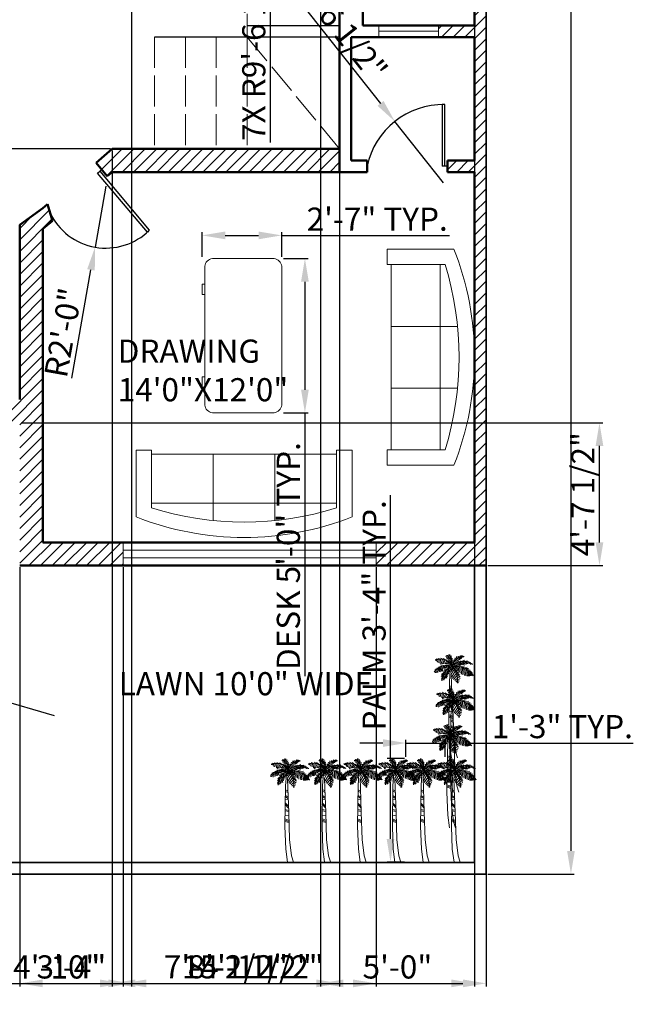
# Model space of a CAD drawing. Units: inches. Extents: x 36184 to 36805, y 18177 to 19069.
# Tile 2 of 5: x 36484 to 36723, y 18177 to 18560. Entities that reach past the tile are written whole.
import ezdxf

# ---------------------------------------------------------------- set-up
doc = ezdxf.new("R2010")
doc.units = ezdxf.units.IN
doc.linetypes.add('ACAD_ISO02W100', pattern=[15, 12, -3])
for name, color, linetype, lineweight in [('A-ANNO-DIMS', 2, 'Continuous', 18), ('A-AREA-IDEN', 7, 'Continuous', 25), ('A-DOOR', 4, 'Continuous', 25), ('A-FLOR-STRS', 7, 'Continuous', 25), ('A-FLOR-STRS-OVHD', 7, 'ACAD_ISO02W100', 18), ('A-FURN', 8, 'Continuous', 18), ('A-GLAZ', 4, 'Continuous', 18), ('A-WALL', 7, 'Continuous', 50), ('C-PROP', 7, 'Continuous', 35), ('L-PLNT', 94, 'Continuous', 13), ('L-SITE-WALL', 7, 'Continuous', 35)]:
    doc.layers.add(name, color=color, linetype=linetype, lineweight=lineweight)
doc.layers.add('A-WALL-PATT', color=244, linetype='Continuous', lineweight=13, true_color=0x991b1e)
doc.styles.get("Standard").update_dxf_attribs({"font": 'arial.ttf'})
doc.dimstyles.new('ISO-25', dxfattribs={"dimtxt": 9, "dimasz": 9, "dimexe": 1.25, "dimexo": 0.625, "dimtad": 1, "dimdec": 1, "dimrnd": 9, "dimlunit": 3, "dimtxsty": 'Standard', "dimcen": 2.5, "dimadec": 0, "dimazin": 0, "dimtfac": 1, "dimtdec": 1, "dimtmove": 0, "dimatfit": 3, "dimfxl": 1, "dimarcsym": 0})

# ---------------------------------------------------------------- blocks, each defined once
blk = doc.blocks.new('Tree - palm elevation')
for p, q in [((-25.283, 191.751), (-29.342, 192.246)), ((-26.443, 191.503), (-26.636, 186.051)), ((-20.064, 191.751), (-25.863, 193.238)), ((-23.737, 191.751), (-24.51, 185.06)), ((-21.031, 191.998), (-21.804, 183.325)), ((-15.232, 191.255), (-20.644, 193.981)), ((-17.551, 191.503), (-20.451, 181.343)), ((-9.433, 189.025), (-15.618, 193.238)), ((-6.727, 197.202), (-11.366, 197.45)), ((-3.441, 194.477), (-10.013, 195.716)), ((-1.894, 192.494), (-9.24, 193.733)), ((-7.5, 199.68), (-7.5, 197.946)), ((-0.541, 189.52), (-7.307, 192.494)), ((-5.567, 196.707), (-4.987, 201.167)), ((-4.407, 195.716), (-3.247, 200.672)), ((-2.474, 193.733), (-1.315, 199.433)), ((-1.121, 190.759), (0.232, 196.955)), ((0.038, 188.281), (1.778, 193.981)), ((5.837, 187.786), (7.577, 194.229)), ((9.317, 191.255), (10.283, 196.955)), ((11.25, 192.494), (15.889, 190.512)), ((11.829, 192.99), (13.182, 197.45)), ((13.956, 194.229), (14.729, 196.955)), ((14.536, 193.981), (17.242, 191.255)), ((15.116, 194.477), (17.822, 198.689)), ((16.082, 194.972), (17.822, 192.494)), ((18.015, 195.716), (20.914, 198.689)), ((18.015, 195.468), (18.981, 192.494)), ((19.368, 196.459), (19.948, 193.733)), ((20.914, 196.459), (21.301, 194.972)), ((21.301, 196.459), (22.847, 198.441)), ((22.074, 196.707), (23.427, 195.716)), ((23.234, 196.707), (23.62, 197.698)), ((-29.729, 190.759), (-31.469, 191.255)), ((-30.309, 190.512), (-30.695, 189.025)), ((-27.409, 173.413), (-30.695, 172.67)), ((-28.763, 190.759), (-28.763, 188.281)), ((-25.09, 175.148), (-28.376, 174.404)), ((-27.989, 172.422), (-26.056, 166.227)), ((-26.829, 173.661), (-23.544, 167.218)), ((-25.476, 174.652), (-21.224, 167.466)), ((-21.031, 177.626), (-24.897, 176.387)), ((-24.317, 175.891), (-18.711, 168.457)), ((-22.191, 176.635), (-16.391, 169.448)), ((-15.618, 179.36), (-20.644, 178.617)), ((-20.064, 177.626), (-15.812, 172.67)), ((-14.265, 190.759), (-18.131, 182.086)), ((-17.358, 178.617), (-13.299, 173.661)), ((-11.753, 189.768), (-15.425, 182.83)), ((-15.038, 179.36), (-10.786, 174.404)), ((-4.214, 175.148), (-14.072, 170.935)), ((-8.08, 188.034), (-12.912, 182.83)), ((-12.332, 180.104), (-9.433, 175.643)), ((-4.987, 185.803), (-10.979, 182.086)), ((-10.206, 180.104), (-8.08, 175.891)), ((-6.147, 186.299), (-9.24, 190.264)), ((-1.701, 176.882), (-8.66, 175.396)), ((-8.273, 180.104), (-6.147, 176.635)), ((-3.247, 183.821), (-8.08, 181.838)), ((-6.92, 172.917), (-5.374, 163.253)), ((-6.34, 179.608), (-4.6, 177.13)), ((-5.76, 190.016), (0.618, 185.308)), ((-5.76, 188.034), (-1.508, 182.582)), ((-1.315, 181.591), (-5.374, 181.095)), ((-4.6, 174.9), (-4.021, 166.722)), ((-4.021, 179.36), (-2.861, 177.378)), ((-2.668, 185.803), (1.198, 181.343)), ((-2.668, 176.387), (-2.376, 170.594)), ((-0.348, 180.352), (-1.894, 180.104)), ((-0.928, 176.882), (-1.508, 173.909)), ((2.551, 175.891), (-0.928, 171.431)), ((3.711, 174.404), (-0.541, 167.961)), ((1.585, 177.13), (0.038, 174.652)), ((1.005, 185.803), (2.358, 190.759)), ((1.005, 182.582), (2.938, 186.547)), ((1.585, 177.13), (6.61, 176.139)), ((2.938, 182.582), (6.61, 183.821)), ((2.938, 175.891), (8.737, 173.413)), ((4.098, 185.06), (4.678, 190.512)), ((4.098, 180.847), (8.35, 179.608)), ((4.291, 173.909), (12.216, 168.953)), ((4.871, 186.051), (10.09, 186.547)), ((4.871, 181.591), (8.544, 184.812)), ((5.644, 181.838), (13.569, 178.865)), ((6.224, 178.121), (8.157, 175.148)), ((6.997, 188.529), (12.216, 187.786)), ((7.384, 178.369), (10.476, 179.36)), ((7.77, 183.325), (16.082, 179.856)), ((8.157, 178.121), (10.476, 172.422)), ((8.544, 190.512), (13.763, 189.52)), ((9.51, 184.317), (15.502, 188.034)), ((10.476, 177.874), (12.796, 169.696)), ((11.25, 184.812), (17.628, 180.352)), ((11.829, 177.874), (18.015, 179.113)), ((13.182, 177.874), (14.729, 166.97)), ((14.536, 185.803), (19.948, 180.847)), ((15.695, 186.299), (19.368, 188.777)), ((15.889, 177.13), (16.855, 164.492)), ((17.242, 186.547), (23.041, 180.599)), ((18.015, 177.13), (26.133, 179.113)), ((18.981, 175.891), (19.561, 163.005)), ((19.368, 187.29), (26.133, 189.768)), ((20.721, 187.042), (25.167, 181.343)), ((20.914, 175.891), (30.966, 176.635)), ((21.688, 175.396), (22.074, 161.518)), ((23.814, 187.29), (26.907, 181.343)), ((23.814, 174.404), (25.554, 160.279)), ((24.78, 187.538), (31.546, 188.777)), ((25.554, 173.661), (33.285, 173.661)), ((26.133, 187.29), (29.419, 181.838)), ((26.52, 173.165), (28.066, 159.784)), ((28.066, 187.29), (30.966, 182.582)), ((29.806, 186.795), (32.319, 183.078)), ((29.999, 186.795), (33.092, 187.29)), ((32.512, 186.299), (35.218, 186.299)), ((33.479, 186.051), (34.445, 182.83)), ((35.605, 185.556), (37.151, 185.308)), ((35.798, 185.308), (36.958, 181.591)), ((38.118, 184.317), (38.504, 181.838)), ((39.857, 182.83), (40.244, 181.591)), ((-32.628, 167.961), (-33.208, 167.961)), ((-32.628, 167.713), (-32.435, 165.979)), ((-28.956, 172.174), (-32.435, 170.192)), ((-31.082, 169.944), (-32.435, 169.2)), ((-31.662, 168.705), (-31.082, 165.483)), ((-29.922, 170.687), (-27.989, 165.235)), ((-14.265, 164.244), (-19.678, 158.049)), ((-16.005, 160.031), (-19.484, 154.084)), ((-18.131, 153.589), (-19.484, 151.606)), ((-12.139, 167.961), (-19.098, 162.014)), ((-17.358, 155.819), (-14.845, 151.358)), ((-8.466, 171.678), (-16.585, 167.713)), ((-16.585, 158.545), (-13.106, 152.35)), ((-15.618, 160.775), (-12.332, 154.332)), ((-14.265, 163.749), (-10.786, 154.828)), ((-12.719, 166.722), (-9.046, 154.828)), ((-10.979, 168.457), (-7.887, 157.801)), ((-8.853, 170.935), (-7.113, 160.527)), ((5.257, 171.926), (-0.155, 163.005)), ((7.384, 168.705), (0.812, 157.553)), ((9.317, 164.244), (2.358, 154.332)), ((10.863, 159.784), (4.484, 152.35)), ((6.417, 170.439), (14.729, 164.492)), ((11.829, 155.075), (6.804, 150.119)), ((8.544, 165.979), (16.662, 160.527)), ((10.09, 162.51), (17.435, 157.058)), ((11.443, 157.553), (16.855, 154.332)), ((28.839, 172.174), (36.378, 170.687)), ((29.226, 171.926), (30.966, 158.545)), ((30.966, 170.687), (38.891, 167.713)), ((32.126, 169.696), (32.512, 158.545)), ((34.058, 168.705), (34.445, 158.545)), ((35.412, 167.713), (41.404, 164.988)), ((36.378, 166.474), (35.605, 158.792)), ((37.731, 165.235), (36.958, 159.288)), ((37.924, 165.235), (41.404, 163.749)), ((38.504, 164.492), (38.504, 159.536)), ((39.664, 163.253), (42.37, 161.766)), ((39.857, 162.757), (39.857, 160.031)), ((40.824, 161.766), (41.21, 160.031)), ((41.21, 161.518), (42.757, 160.279)), ((-17.938, 152.597), (-16.972, 151.111)), ((-4.081, 140.645), (0.753, 138.261)), ((-4.081, 137.547), (0.753, 135.163)), ((12.603, 151.111), (8.544, 148.385)), ((12.216, 148.137), (10.09, 147.393)), ((12.409, 145.659), (11.056, 145.659)), ((12.216, 153.093), (16.082, 151.606)), ((12.409, 146.898), (13.763, 146.402)), ((12.603, 149.872), (15.116, 149.128)), ((-4.081, 129.205), (1.124, 126.821)), ((-4.081, 127.298), (1.31, 123.246)), ((-4.081, 121.578), (1.31, 120.863)), ((-4.639, 102.273), (1.868, 100.604)), ((-4.453, 112.283), (1.682, 105.133)), ((-4.453, 99.651), (2.24, 98.459)), ((-4.267, 114.428), (1.682, 108.708)), ((-4.825, 83.921), (2.612, 81.061)), ((-4.639, 81.299), (2.797, 78.916)), ((-4.639, 78.916), (2.797, 76.771)), ((-4.453, 91.071), (2.426, 89.641))]:
    blk.add_line(p, q)
for points in [[(-2.363, 170.553), (-3.88, 148.505), (-4.988, 69.634), (-3.325, 24.869), (0, 0)], [(-0.116, 162.848), (0.554, 143.532), (2.217, 96.635), (3.88, 44.054), (7.76, 12.079), (11.64, 0)]]:
    blk.add_lwpolyline(points)
for centre, radius, start, end in [((-21.738, 166.094), 25.899, 27.67115, 112.5305), ((-18.427, 181.448), 19.715, 350.285, 64.11229), ((25.595, 171.567), 25.395, 91.40319, 163.882), ((-9.259, 151.732), 28.386, 68.38311, 147.5322), ((14.394, 148.393), 32.752, 113.7592, 177.4133), ((23.687, 155.341), 32.188, 56.19272, 134.3213), ((5.828, 132.718), 45.639, 35.98777, 95.82273), ((-32.8, 147.923), 45.309, 356.1943, 41.37848)]:
    blk.add_arc(centre, radius, start, end)
blk = doc.blocks.new('Sofa - Roundback 7 ft.')
for p, q in [((-12.00002, -32.4421), (-12.00003, -6.5971)), ((11.99997, -32.4421), (11.99998, -6.5971)), ((-36.000027, -34), (-36.000027, -11.4696)), ((35.99998, -34), (35.99998, -11.4696)), ((-35.999844, -13.3819), (35.9998, -13.3819)), ((-36.000027, -32.4421), (35.99998, -32.4421))]:
    blk.add_line(p, q)
for points in [[(-36.000027, -34), (-42.000027, -34), (-42.000027, -8)], [(41.99998, -8), (41.99998, -34), (35.99998, -34)]]:
    blk.add_lwpolyline(points)
for centre, radius, start, end in [((0, -114.25), 114.25, 68.43141, 111.5686), ((-0.00001, -127.1968), 121.1968, 72.72033, 107.2797)]:
    blk.add_arc(centre, radius, start, end)
blk = doc.blocks.new('Desk - 30 x 60 in.')
for p, q in [((-26.999995, 0), (26.999995, 0)), ((-29.999995, -27), (-29.999995, -3)), ((29.999995, -3), (29.999995, -27)), ((26.999995, -30), (-26.999995, -30)), ((-20.000005, -30), (-20.000005, -31)), ((-16.000005, -31), (-16.000005, -30)), ((15.999995, -31), (15.999995, -30)), ((19.999995, -30), (19.999995, -31)), ((-20.000005, -31), (-16.000005, -31)), ((19.999995, -31), (15.999995, -31))]:
    blk.add_line(p, q)
for centre, start, end in [((-26.499995, -3.5), 98.1301, 171.8699), ((26.499995, -3.5), 8.130102, 81.8699), ((-26.499995, -26.5), 188.1301, 261.8699), ((26.499995, -26.5), 278.1301, 351.8699)]:
    blk.add_arc(centre, 3.535534, start, end)
blk = doc.blocks.new('*D15')
at = {"layer": 'A-ANNO-DIMS', "color": 0, "lineweight": -2, "transparency": 16777216}
for p, q in [((36665.94, 19007.3), (36699.58, 19007.3)), ((36698.33, 18998.3), (36698.33, 18236.3)), ((36665.94, 18227.3), (36699.58, 18227.3))]:
    blk.add_line(p, q, dxfattribs=at)
at = {"layer": 'A-ANNO-DIMS', "color": 0, "transparency": 16777216}
for points in [[(36696.83, 18998.3), (36699.83, 18998.3), (36698.33, 19007.3)], [(36696.83, 18236.3), (36699.83, 18236.3), (36698.33, 18227.3)]]:
    blk.add_solid(points, dxfattribs=at)
at = {"layer": 'Defpoints', "color": 0, "transparency": 16777216}
for p in [(36665.31, 19007.3), (36665.31, 18227.3), (36698.33, 18227.3)]:
    blk.add_point(p, dxfattribs=at)
at = {"layer": 'A-ANNO-DIMS', "color": 0, "transparency": 16777216, "insert": (36693.1, 18617.3), "char_height": 9, "attachment_point": 5, "rotation": 90}
blk.add_mtext('65\'-3"', dxfattribs=at)
blk = doc.blocks.new('DOOR-LEAF-24IN')
for p, q in [((1, 0), (1, 24)), ((1, 24), (2, 24)), ((2, 24), (2, 0)), ((0, 0), (1, 0)), ((1, 0), (2, 0))]:
    blk.add_line(p, q)
blk = doc.blocks.new('*D20')
at = {"layer": 'A-ANNO-DIMS', "color": 0, "lineweight": -2, "transparency": 16777216}
for p, q in [((36628.11, 18272.22), (36628.11, 18374.61)), ((36633.52, 18272.22), (36626.86, 18272.22)), ((36628.11, 18240.99), (36628.11, 18263.22)), ((36633.52, 18231.99), (36626.86, 18231.99))]:
    blk.add_line(p, q, dxfattribs=at)
at = {"layer": 'A-ANNO-DIMS', "color": 0, "transparency": 16777216}
for points in [[(36626.61, 18263.22), (36629.61, 18263.22), (36628.11, 18272.22)], [(36626.61, 18240.99), (36629.61, 18240.99), (36628.11, 18231.99)]]:
    blk.add_solid(points, dxfattribs=at)
at = {"layer": 'Defpoints', "color": 0, "transparency": 16777216}
for p in [(36628.11, 18272.22), (36634.14, 18272.22), (36634.14, 18231.99)]:
    blk.add_point(p, dxfattribs=at)
at = {"layer": 'A-ANNO-DIMS', "color": 0, "transparency": 16777216, "insert": (36622.88, 18327.92), "char_height": 9, "attachment_point": 5, "rotation": 90}
blk.add_mtext('PALM 3\'-4" TYP.', dxfattribs=at)
blk = doc.blocks.new('*D21')
at = {"layer": 'A-ANNO-DIMS', "color": 0, "lineweight": -2, "transparency": 16777216}
for p, q in [((36634.14, 18272.85), (36634.14, 18279.51)), ((36649.34, 18272.85), (36649.34, 18279.51)), ((36625.14, 18278.26), (36616.14, 18278.26)), ((36634.14, 18278.26), (36649.34, 18278.26)), ((36658.34, 18278.26), (36722.6, 18278.26))]:
    blk.add_line(p, q, dxfattribs=at)
at = {"layer": 'A-ANNO-DIMS', "color": 0, "transparency": 16777216}
for points in [[(36625.14, 18279.76), (36625.14, 18276.76), (36634.14, 18278.26)], [(36658.34, 18279.76), (36658.34, 18276.76), (36649.34, 18278.26)]]:
    blk.add_solid(points, dxfattribs=at)
at = {"layer": 'Defpoints', "color": 0, "transparency": 16777216}
for p in [(36649.34, 18278.26), (36634.14, 18272.22), (36649.34, 18272.22)]:
    blk.add_point(p, dxfattribs=at)
at = {"layer": 'A-ANNO-DIMS', "color": 0, "transparency": 16777216, "insert": (36694.97, 18283.48), "char_height": 9, "attachment_point": 5}
blk.add_mtext('1\'-3" TYP.', dxfattribs=at)
blk = doc.blocks.new('*D38')
at = {"layer": 'A-ANNO-DIMS', "color": 0, "lineweight": -2, "transparency": 16777216}
for p, q in [((36586.42, 18466.67), (36596.05, 18466.67)), ((36594.8, 18457.67), (36594.8, 18415.67)), ((36586.42, 18406.67), (36596.05, 18406.67)), ((36594.8, 18406.67), (36594.8, 18304.28))]:
    blk.add_line(p, q, dxfattribs=at)
at = {"layer": 'A-ANNO-DIMS', "color": 0, "transparency": 16777216}
for points in [[(36593.3, 18457.67), (36596.3, 18457.67), (36594.8, 18466.67)], [(36593.3, 18415.67), (36596.3, 18415.67), (36594.8, 18406.67)]]:
    blk.add_solid(points, dxfattribs=at)
at = {"layer": 'Defpoints', "color": 0, "transparency": 16777216}
for p in [(36585.8, 18466.67), (36585.8, 18406.67), (36594.8, 18406.67)]:
    blk.add_point(p, dxfattribs=at)
at = {"layer": 'A-ANNO-DIMS', "color": 0, "transparency": 16777216, "insert": (36589.52, 18350.97), "char_height": 9, "attachment_point": 5, "rotation": 90}
blk.add_mtext('DESK 5\'-0" TYP.', dxfattribs=at)
blk = doc.blocks.new('*D39')
at = {"layer": 'A-ANNO-DIMS', "color": 0, "lineweight": -2, "transparency": 16777216}
for p, q in [((36554.8, 18467.29), (36554.8, 18476.92)), ((36563.8, 18475.67), (36576.8, 18475.67)), ((36585.8, 18467.29), (36585.8, 18476.92)), ((36585.8, 18475.67), (36651.06, 18475.67))]:
    blk.add_line(p, q, dxfattribs=at)
at = {"layer": 'A-ANNO-DIMS', "color": 0, "transparency": 16777216}
for points in [[(36563.8, 18477.17), (36563.8, 18474.17), (36554.8, 18475.67)], [(36576.8, 18477.17), (36576.8, 18474.17), (36585.8, 18475.67)]]:
    blk.add_solid(points, dxfattribs=at)
at = {"layer": 'Defpoints', "color": 0, "transparency": 16777216}
for p in [(36585.8, 18475.67), (36554.8, 18466.67), (36585.8, 18466.67)]:
    blk.add_point(p, dxfattribs=at)
at = {"layer": 'A-ANNO-DIMS', "color": 0, "transparency": 16777216, "insert": (36622.93, 18480.82), "char_height": 9, "attachment_point": 5}
blk.add_mtext('2\'-7" TYP.', dxfattribs=at)
blk = doc.blocks.new('*D46')
at = {"layer": 'A-ANNO-DIMS', "color": 0, "lineweight": -2, "transparency": 16777216}
for p, q in [((36519.81, 18508.68), (36519.81, 18183.55)), ((36608.31, 18508.68), (36608.31, 18183.55)), ((36528.81, 18184.8), (36599.31, 18184.8))]:
    blk.add_line(p, q, dxfattribs=at)
at = {"layer": 'A-ANNO-DIMS', "color": 0, "transparency": 16777216}
for points in [[(36528.81, 18186.3), (36528.81, 18183.3), (36519.81, 18184.8)], [(36599.31, 18186.3), (36599.31, 18183.3), (36608.31, 18184.8)]]:
    blk.add_solid(points, dxfattribs=at)
at = {"layer": 'Defpoints', "color": 0, "transparency": 16777216}
for p in [(36519.81, 18509.3), (36608.31, 18509.3), (36608.31, 18184.8)]:
    blk.add_point(p, dxfattribs=at)
at = {"layer": 'A-ANNO-DIMS', "color": 0, "transparency": 16777216, "insert": (36564.06, 18190.08), "char_height": 9, "attachment_point": 5}
blk.add_mtext('7\'-4 1/2"', dxfattribs=at)
blk = doc.blocks.new('*D47')
at = {"layer": 'A-ANNO-DIMS', "color": 0, "lineweight": -2, "transparency": 16777216}
for p, q in [((36519.19, 18608.3), (36201.56, 18608.3)), ((36202.81, 18518.3), (36202.81, 18599.3)), ((36519.19, 18509.3), (36201.56, 18509.3))]:
    blk.add_line(p, q, dxfattribs=at)
at = {"layer": 'A-ANNO-DIMS', "color": 0, "transparency": 16777216}
for points in [[(36201.31, 18599.3), (36204.31, 18599.3), (36202.81, 18608.3)], [(36201.31, 18518.3), (36204.31, 18518.3), (36202.81, 18509.3)]]:
    blk.add_solid(points, dxfattribs=at)
at = {"layer": 'Defpoints', "color": 0, "transparency": 16777216}
for p in [(36202.81, 18608.3), (36519.81, 18608.3), (36519.81, 18509.3)]:
    blk.add_point(p, dxfattribs=at)
at = {"layer": 'A-ANNO-DIMS', "color": 0, "transparency": 16777216, "insert": (36197.59, 18558.8), "char_height": 9, "attachment_point": 5, "rotation": 90}
blk.add_mtext('8\'-3"', dxfattribs=at)
blk = doc.blocks.new('*D48')
at = {"layer": 'A-ANNO-DIMS', "color": 0, "lineweight": -2, "transparency": 16777216}
for p, q in [((36600.81, 18829.68), (36600.81, 18183.55)), ((36660.81, 18829.68), (36660.81, 18183.55)), ((36609.81, 18184.8), (36651.81, 18184.8))]:
    blk.add_line(p, q, dxfattribs=at)
at = {"layer": 'A-ANNO-DIMS', "color": 0, "transparency": 16777216}
for points in [[(36609.81, 18186.3), (36609.81, 18183.3), (36600.81, 18184.8)], [(36651.81, 18186.3), (36651.81, 18183.3), (36660.81, 18184.8)]]:
    blk.add_solid(points, dxfattribs=at)
at = {"layer": 'Defpoints', "color": 0, "transparency": 16777216}
for p in [(36600.81, 18830.3), (36660.81, 18830.3), (36660.81, 18184.8)]:
    blk.add_point(p, dxfattribs=at)
at = {"layer": 'A-ANNO-DIMS', "color": 0, "transparency": 16777216, "insert": (36630.81, 18190.02), "char_height": 9, "attachment_point": 5}
blk.add_mtext('5\'-0"', dxfattribs=at)
blk = doc.blocks.new('*D51')
at = {"layer": 'A-ANNO-DIMS', "color": 0, "lineweight": -2, "transparency": 16777216}
for p, q in [((36483.81, 18346.68), (36483.81, 18183.55)), ((36665.31, 18346.68), (36665.31, 18183.55)), ((36492.81, 18184.8), (36656.31, 18184.8))]:
    blk.add_line(p, q, dxfattribs=at)
at = {"layer": 'A-ANNO-DIMS', "color": 0, "transparency": 16777216}
for points in [[(36492.81, 18186.3), (36492.81, 18183.3), (36483.81, 18184.8)], [(36656.31, 18186.3), (36656.31, 18183.3), (36665.31, 18184.8)]]:
    blk.add_solid(points, dxfattribs=at)
at = {"layer": 'Defpoints', "color": 0, "transparency": 16777216}
for p in [(36483.81, 18347.3), (36665.31, 18347.3), (36665.31, 18184.8)]:
    blk.add_point(p, dxfattribs=at)
at = {"layer": 'A-ANNO-DIMS', "color": 0, "transparency": 16777216, "insert": (36574.56, 18190.08), "char_height": 9, "attachment_point": 5}
blk.add_mtext('15\'-1 1/2"', dxfattribs=at)
blk = doc.blocks.new('*D52')
at = {"layer": 'A-ANNO-DIMS', "color": 0, "lineweight": -2, "transparency": 16777216}
for p, q in [((36484.44, 18402.8), (36710.68, 18402.8)), ((36709.43, 18356.3), (36709.43, 18393.8)), ((36665.94, 18347.3), (36710.68, 18347.3))]:
    blk.add_line(p, q, dxfattribs=at)
at = {"layer": 'A-ANNO-DIMS', "color": 0, "transparency": 16777216}
for points in [[(36707.93, 18393.8), (36710.93, 18393.8), (36709.43, 18402.8)], [(36707.93, 18356.3), (36710.93, 18356.3), (36709.43, 18347.3)]]:
    blk.add_solid(points, dxfattribs=at)
at = {"layer": 'Defpoints', "color": 0, "transparency": 16777216}
for p in [(36483.81, 18402.8), (36709.43, 18402.8), (36665.31, 18347.3)]:
    blk.add_point(p, dxfattribs=at)
at = {"layer": 'A-ANNO-DIMS', "color": 0, "transparency": 16777216, "insert": (36704.15, 18375.05), "char_height": 9, "attachment_point": 5, "rotation": 90}
blk.add_mtext('4\'-7 1/2"', dxfattribs=at)
blk = doc.blocks.new('*D57')
at = {"layer": 'A-ANNO-DIMS', "color": 0, "lineweight": -2, "transparency": 16777216}
for p, q in [((36524.04, 18346.68), (36524.04, 18183.55)), ((36622.58, 18346.68), (36622.58, 18183.55)), ((36533.04, 18184.8), (36613.58, 18184.8))]:
    blk.add_line(p, q, dxfattribs=at)
at = {"layer": 'A-ANNO-DIMS', "color": 0, "transparency": 16777216}
for points in [[(36533.04, 18186.3), (36533.04, 18183.3), (36524.04, 18184.8)], [(36613.58, 18186.3), (36613.58, 18183.3), (36622.58, 18184.8)]]:
    blk.add_solid(points, dxfattribs=at)
at = {"layer": 'Defpoints', "color": 0, "transparency": 16777216}
for p in [(36524.04, 18347.3), (36622.58, 18347.3), (36622.58, 18184.8)]:
    blk.add_point(p, dxfattribs=at)
at = {"layer": 'A-ANNO-DIMS', "color": 0, "transparency": 16777216, "insert": (36573.31, 18190.08), "char_height": 9, "attachment_point": 5}
blk.add_mtext('8\'-2 1/2"', dxfattribs=at)
blk = doc.blocks.new('*D58')
at = {"layer": 'A-ANNO-DIMS', "color": 0, "lineweight": -2, "transparency": 16777216}
for p, q in [((36483.81, 18346.68), (36483.81, 18183.55)), ((36524.04, 18346.68), (36524.04, 18183.55)), ((36492.81, 18184.8), (36515.04, 18184.8))]:
    blk.add_line(p, q, dxfattribs=at)
at = {"layer": 'A-ANNO-DIMS', "color": 0, "transparency": 16777216}
for points in [[(36492.81, 18186.3), (36492.81, 18183.3), (36483.81, 18184.8)], [(36515.04, 18186.3), (36515.04, 18183.3), (36524.04, 18184.8)]]:
    blk.add_solid(points, dxfattribs=at)
at = {"layer": 'Defpoints', "color": 0, "transparency": 16777216}
for p in [(36483.81, 18347.3), (36524.04, 18347.3), (36524.04, 18184.8)]:
    blk.add_point(p, dxfattribs=at)
at = {"layer": 'A-ANNO-DIMS', "color": 0, "transparency": 16777216, "insert": (36503.92, 18190.03), "char_height": 9, "attachment_point": 5}
blk.add_mtext('3\'-4"', dxfattribs=at)
blk = doc.blocks.new('*D59')
at = {"layer": 'A-ANNO-DIMS', "color": 0, "lineweight": -2, "transparency": 16777216}
for p, q in [((36469.15, 18918.18), (36469.15, 18183.55)), ((36527.35, 18918.18), (36527.35, 18183.55)), ((36478.15, 18184.8), (36518.35, 18184.8))]:
    blk.add_line(p, q, dxfattribs=at)
at = {"layer": 'A-ANNO-DIMS', "color": 0, "transparency": 16777216}
for points in [[(36478.15, 18186.3), (36478.15, 18183.3), (36469.15, 18184.8)], [(36518.35, 18186.3), (36518.35, 18183.3), (36527.35, 18184.8)]]:
    blk.add_solid(points, dxfattribs=at)
at = {"layer": 'Defpoints', "color": 0, "transparency": 16777216}
for p in [(36469.15, 18918.8), (36527.35, 18918.8), (36527.35, 18184.8)]:
    blk.add_point(p, dxfattribs=at)
at = {"layer": 'A-ANNO-DIMS', "color": 0, "transparency": 16777216, "insert": (36498.25, 18190.02), "char_height": 9, "attachment_point": 5}
blk.add_mtext('4\'-10"', dxfattribs=at)
blk = doc.blocks.new('*D61')
at = {"layer": 'A-ANNO-DIMS', "color": 0, "lineweight": -2, "transparency": 16777216}
for p, q in [((36364.63, 18327.57), (36432.54, 18307.73)), ((36497.33, 18288.82), (36441.18, 18305.21))]:
    blk.add_line(p, q, dxfattribs=at)
at = {"layer": 'A-ANNO-DIMS', "color": 0, "transparency": 16777216}
blk.add_solid([(36432.97, 18309.17), (36432.12, 18306.29), (36441.18, 18305.21)], dxfattribs=at)
at = {"layer": 'Defpoints', "color": 0, "transparency": 16777216}
for p in [(36441.18, 18305.21), (36497.33, 18288.82)]:
    blk.add_point(p, dxfattribs=at)
at = {"layer": 'A-ANNO-DIMS', "color": 0, "transparency": 16777216, "insert": (36395.75, 18323.98), "char_height": 9, "attachment_point": 5, "rotation": 343.7204}
blk.add_mtext('R4\'-10 1/2"', dxfattribs=at)
blk = doc.blocks.new('*D65')
at = {"layer": 'A-ANNO-DIMS', "color": 0, "lineweight": -2, "transparency": 16777216}
for p, q in [((36584.61, 18576.97), (36624.23, 18527.01)), ((36648.74, 18496.11), (36629.82, 18519.96))]:
    blk.add_line(p, q, dxfattribs=at)
at = {"layer": 'A-ANNO-DIMS', "color": 0, "transparency": 16777216}
blk.add_solid([(36625.4, 18527.95), (36623.05, 18526.08), (36629.82, 18519.96)], dxfattribs=at)
at = {"layer": 'Defpoints', "color": 0, "transparency": 16777216}
for p in [(36629.82, 18519.96), (36648.74, 18496.11)]:
    blk.add_point(p, dxfattribs=at)
at = {"layer": 'A-ANNO-DIMS', "color": 0, "transparency": 16777216, "insert": (36605.76, 18558.8), "char_height": 9, "attachment_point": 5, "rotation": 308.4188}
blk.add_mtext('R2\'-6 1/2"', dxfattribs=at)
blk = doc.blocks.new('*D69')
at = {"layer": 'A-ANNO-DIMS', "color": 0, "lineweight": -2, "transparency": 16777216}
for p, q in [((36517.35, 18494.76), (36513.14, 18471.1)), ((36504.07, 18420.12), (36511.56, 18462.24))]:
    blk.add_line(p, q, dxfattribs=at)
at = {"layer": 'A-ANNO-DIMS', "color": 0, "transparency": 16777216}
blk.add_solid([(36510.08, 18462.51), (36513.04, 18461.98), (36513.14, 18471.1)], dxfattribs=at)
at = {"layer": 'Defpoints', "color": 0, "transparency": 16777216}
for p in [(36517.35, 18494.76), (36513.14, 18471.1)]:
    blk.add_point(p, dxfattribs=at)
at = {"layer": 'A-ANNO-DIMS', "color": 0, "transparency": 16777216, "insert": (36501.89, 18437.66), "char_height": 9, "attachment_point": 5, "rotation": 79.9104}
blk.add_mtext('R2\'-0"', dxfattribs=at)
blk = doc.blocks.new('*D71')
at = {"layer": 'A-ANNO-DIMS', "color": 0, "lineweight": -2, "transparency": 16777216}
for p, q in [((36581.36, 18731.55), (36581.36, 18617.3)), ((36581.36, 18511.74), (36581.36, 18608.3))]:
    blk.add_line(p, q, dxfattribs=at)
at = {"layer": 'A-ANNO-DIMS', "color": 0, "transparency": 16777216}
blk.add_solid([(36579.86, 18608.3), (36582.86, 18608.3), (36581.36, 18617.3)], dxfattribs=at)
at = {"layer": 'Defpoints', "color": 0, "transparency": 16777216}
for p in [(36581.36, 18731.55), (36581.36, 18617.3)]:
    blk.add_point(p, dxfattribs=at)
at = {"layer": 'A-ANNO-DIMS', "color": 0, "transparency": 16777216, "insert": (36576.08, 18548.75), "char_height": 9, "attachment_point": 5, "rotation": 90}
blk.add_mtext('7X R9\'-6 1/2"', dxfattribs=at)

msp = doc.modelspace()

# ---------------------------------------------------------------- hatches: boundary and pattern name
at = {"layer": 'A-WALL-PATT'}
h = msp.add_hatch(dxfattribs=at)
h.set_pattern_fill('ANSI31', color=256)
h.paths.add_polyline_path([(36318.81, 18555.8), (36459.81, 18555.8), (36459.81, 18705.8), (36440.41, 18705.8), (36440.41, 18696.8), (36450.81, 18696.8), (36450.81, 18564.8), (36318.81, 18564.8), (36318.81, 18591.83), (36309.81, 18591.83), (36309.81, 18525.65), (36318.81, 18525.65)], flags=17)
h.paths.add_polyline_path([(36318.81, 18455.41), (36309.81, 18455.41), (36309.81, 18402.8), (36338.76, 18402.8), (36338.76, 18411.8), (36318.81, 18411.8)], flags=17)
h.paths.add_polyline_path([(36423.09, 18411.8), (36400.25, 18411.8), (36400.25, 18402.8), (36423.09, 18402.8)], flags=17)
h.paths.add_polyline_path([(36492.81, 18478.27), (36496.58, 18481.34), (36494.6, 18487.78), (36492.81, 18486.25), (36483.81, 18479.84), (36483.81, 18411.8), (36473.38, 18411.8), (36473.38, 18402.8), (36483.81, 18402.8), (36483.81, 18356.3), (36483.81, 18347.3), (36519.81, 18347.3), (36524.04, 18347.3), (36524.04, 18356.3), (36492.81, 18356.3)], flags=17)
h.paths.add_polyline_path([(36665.31, 18608.3), (36660.81, 18608.3), (36660.81, 18557.3), (36646.76, 18557.3), (36646.76, 18552.8), (36660.81, 18552.8), (36660.81, 18504.8), (36650.24, 18504.8), (36650.24, 18500.3), (36660.81, 18500.3), (36660.81, 18356.3), (36622.58, 18356.3), (36622.58, 18347.3), (36665.31, 18347.3)])
h.paths.add_polyline_path([(36608.31, 18509.3), (36519.81, 18509.3), (36513.55, 18503.95), (36517.84, 18498.69), (36519.81, 18500.3), (36608.31, 18500.3)])
h.paths.add_polyline_path([(36254.31, 18411.79), (36249.81, 18411.79), (36249.81, 19002.8), (36553.31, 19002.8), (36553.31, 19007.3), (36245.31, 19007.3), (36245.31, 18288.82), (36254.31, 18288.82)])
h.paths.add_polyline_path([(36342.97, 18918.8), (36309.81, 18918.8), (36309.81, 18747.12), (36314.31, 18747.12), (36314.31, 18765.8), (36384.81, 18765.8), (36384.81, 18701.3), (36350.57, 18701.3), (36350.57, 18696.8), (36396.53, 18696.8), (36396.53, 18705.8), (36389.31, 18705.8), (36389.31, 18761.3), (36393.31, 18761.3), (36393.31, 18770.3), (36384.81, 18770.3), (36318.81, 18770.3), (36318.81, 18909.8), (36342.97, 18909.8)], flags=17)
h.paths.add_polyline_path([(36469.15, 18918.8), (36403.35, 18918.8), (36403.35, 18909.8), (36434.31, 18909.8), (36434.31, 18770.3), (36431, 18770.3), (36431, 18761.3), (36449.29, 18761.3), (36449.29, 18770.3), (36443.31, 18770.3), (36443.31, 18909.8), (36469.15, 18909.8)], flags=17)
h.paths.add_polyline_path([(36557.81, 18953.44), (36553.31, 18953.44), (36553.31, 18918.8), (36527.35, 18918.8), (36527.35, 18909.8), (36553.31, 18909.8), (36562.16, 18909.8), (36562.16, 18914.3), (36557.81, 18914.3)])
h.paths.add_polyline_path([(36665.31, 19007.3), (36553.31, 19007.3), (36553.31, 19002.8), (36553.31, 18989.93), (36557.81, 18989.93), (36557.81, 19002.8), (36660.81, 19002.8), (36660.81, 18765.8), (36656.73, 18765.8), (36656.73, 18761.3), (36660.81, 18761.3), (36660.81, 18617.3), (36654.49, 18617.3), (36654.49, 18608.3), (36665.31, 18608.3)])
h.paths.add_polyline_path([(36600.81, 18890.3), (36596.31, 18890.3), (36596.31, 18770.3), (36487.63, 18770.3), (36487.63, 18761.3), (36519.81, 18761.3), (36519.81, 18756.26), (36528.81, 18756.26), (36528.81, 18761.3), (36634.81, 18761.3), (36634.81, 18765.8), (36600.81, 18765.8), (36600.81, 18825.8), (36660.81, 18825.8), (36660.81, 18830.3), (36600.81, 18830.3)])
h.paths.add_polyline_path([(36600.81, 18914.3), (36596.31, 18914.3), (36591.43, 18914.3), (36591.43, 18909.8), (36596.31, 18909.8), (36596.31, 18890.3), (36660.81, 18890.3), (36660.81, 18894.8), (36600.81, 18894.8)], flags=17)
h.paths.add_polyline_path([(36623.57, 18617.3), (36528.81, 18617.3), (36528.81, 18717.38), (36519.81, 18717.38), (36519.81, 18608.3), (36608.31, 18608.3), (36608.31, 18603.13), (36617.31, 18603.13), (36617.31, 18608.3), (36623.57, 18608.3)])
h.paths.add_polyline_path([(36602.02, 18898.95), (36663.11, 18898.95), (36663.11, 18913.37), (36602.02, 18913.37)], flags=25)

# ---------------------------------------------------------------- linework, layer by layer
at = {"layer": 'A-DOOR'}
for p, q in [((36514.11, 18499.89), (36514.98, 18500.62)), ((36533.53, 18476.99), (36514.11, 18499.89)), ((36515.69, 18501.32), (36514.95, 18500.65)), ((36514.95, 18500.65), (36534.25, 18477.68)), ((36534.25, 18477.68), (36533.53, 18476.99))]:
    msp.add_line(p, q, dxfattribs=at)
for centre, radius, start, end in [((36648.74, 18496.11), 30.45, 89.0592, 167.7772), ((36517.35, 18494.76), 24.03, 205.121, 314.7018)]:
    msp.add_arc(centre, radius, start, end, dxfattribs=at)
at = {"layer": 'A-FLOR-STRS'}
for p, q in [((36572.31, 18557.3), (36608.31, 18557.3)), ((36608.31, 18552.8), (36536.31, 18552.8))]:
    msp.add_line(p, q, dxfattribs=at)
at = {"layer": 'A-FLOR-STRS-OVHD'}
for p, q in [((36572.31, 18552.8), (36572.31, 18561.8)), ((36536.31, 18552.8), (36536.31, 18509.3)), ((36548.31, 18552.8), (36548.31, 18509.3)), ((36560.31, 18552.8), (36560.31, 18509.3)), ((36572.31, 18552.8), (36572.31, 18509.3)), ((36572.31, 18552.8), (36608.31, 18509.3))]:
    msp.add_line(p, q, dxfattribs=at)
at = {"layer": 'A-GLAZ'}
for p, q in [((36623.51, 18557.3), (36623.51, 18552.8)), ((36646.76, 18555.05), (36623.51, 18555.05)), ((36646.76, 18557.3), (36646.76, 18552.8)), ((36524.04, 18356.3), (36524.04, 18347.3)), ((36622.58, 18356.3), (36622.58, 18347.3)), ((36622.58, 18353.3), (36524.04, 18353.3)), ((36622.58, 18350.3), (36524.04, 18350.3))]:
    msp.add_line(p, q, dxfattribs=at)
at = {"layer": 'A-WALL'}
for p, q in [((36608.31, 18557.3), (36608.31, 18608.3)), ((36617.31, 18557.3), (36617.31, 18608.3)), ((36660.81, 18557.3), (36660.81, 18608.3)), ((36608.31, 18552.8), (36608.31, 18557.3)), ((36660.81, 18557.3), (36617.31, 18557.3)), ((36608.31, 18500.3), (36608.31, 18552.8)), ((36660.81, 18552.8), (36612.81, 18552.8)), ((36612.81, 18504.8), (36612.81, 18552.8)), ((36660.81, 18504.8), (36660.81, 18552.8)), ((36519.81, 18509.3), (36513.55, 18503.95)), ((36608.31, 18509.3), (36519.81, 18509.3)), ((36513.55, 18503.95), (36517.84, 18498.69)), ((36612.81, 18504.8), (36618.98, 18504.8)), ((36618.98, 18504.8), (36618.98, 18500.3)), ((36650.24, 18504.8), (36650.24, 18500.3)), ((36650.24, 18504.8), (36660.81, 18504.8)), ((36519.81, 18500.3), (36517.84, 18498.69)), ((36612.81, 18500.3), (36519.81, 18500.3)), ((36612.81, 18500.3), (36618.98, 18500.3)), ((36650.24, 18500.3), (36660.81, 18500.3)), ((36660.81, 18356.3), (36660.81, 18500.3)), ((36492.81, 18486.25), (36483.81, 18479.84)), ((36494.6, 18487.78), (36492.81, 18486.25)), ((36494.6, 18487.78), (36496.58, 18481.34)), ((36483.81, 18411.8), (36483.81, 18479.84)), ((36496.58, 18481.34), (36492.81, 18478.27)), ((36492.81, 18356.3), (36492.81, 18478.27)), ((36660.81, 18356.3), (36492.81, 18356.3)), ((36519.81, 18347.3), (36483.81, 18347.3)), ((36665.31, 18347.3), (36519.81, 18347.3))]:
    msp.add_line(p, q, dxfattribs=at)
at = {"layer": 'C-PROP'}
for p, q in [((36665.31, 18227.3), (36665.31, 19007.3)), ((36245.31, 18227.3), (36665.31, 18227.3))]:
    msp.add_line(p, q, dxfattribs=at)
at = {"layer": 'L-SITE-WALL'}
for p, q in [((36660.81, 18231.8), (36660.81, 18347.3)), ((36455.31, 18231.8), (36660.81, 18231.8))]:
    msp.add_line(p, q, dxfattribs=at)

# ---------------------------------------------------------------- block references
at = {"layer": 'A-DOOR', "extrusion": (0, 0, -1), "zscale": -1}
msp.add_blockref('DOOR-LEAF-24IN', (-36650.24, 18502.55), dxfattribs=at)
at = {"layer": 'A-FURN'}
for name, p, rotation in [('Sofa - Roundback 7 ft.', (36660.81, 18428.3), 270), ('Desk - 30 x 60 in.', (36585.8, 18436.67), 270), ('Sofa - Roundback 7 ft.', (36571.14, 18358.21), 180)]:
    msp.add_blockref(name, p, dxfattribs=dict(at, rotation=rotation))
at = {"layer": 'L-PLNT', "xscale": 0.2, "yscale": 0.2}
for p in [(36651.79, 18272.5), (36652.39, 18259.2), (36651.04, 18245.28), (36588.05, 18231.96), (36602.47, 18232), (36616.29, 18231.99), (36629.85, 18231.99), (36640.78, 18231.99), (36652.83, 18231.99)]:
    msp.add_blockref('Tree - palm elevation', p, dxfattribs=at)

# ---------------------------------------------------------------- texts
at = {"layer": 'A-AREA-IDEN', "char_height": 9, "attachment_point": 1}
for s, width, insert in [('DRAWING\\P14\'0"X12\'0"', 107.0089, (36521.96, 18435.16)), ('LAWN 10\'0" WIDE', 168.5618, (36522.33, 18305.83))]:
    msp.add_mtext_dynamic_manual_height_columns(s, width=width, gutter_width=12.5, heights=[0], dxfattribs=dict(at, insert=insert))

# ---------------------------------------------------------------- dimensions: what is measured, and where the dimension line sits
at = {"layer": 'A-ANNO-DIMS'}
for base, p1, p2, override, picture, middle in [((36698.33, 18227.3), (36665.31, 19007.3), (36665.31, 18227.3), {"dimclrd": 0, "dimclre": 0, "dimclrt": 0}, '*D15', (36693.1, 18617.3)), ((36202.81, 18608.3), (36519.81, 18509.3), (36519.81, 18608.3), {"dimdec": 1, "dimlfac": 1, "dimrnd": 0, "dimzin": 1, "dimdsep": 46, "dimlunit": 4, "dimfrac": 2}, '*D47', (36197.59, 18558.8)), ((36709.43, 18402.8), (36665.31, 18347.3), (36483.81, 18402.8), {"dimdec": 1, "dimlfac": 1, "dimrnd": 0, "dimzin": 1, "dimdsep": 46, "dimlunit": 4, "dimfrac": 2}, '*D52', (36704.15, 18375.05))]:
    dim = msp.add_linear_dim(base=base, p1=p1, p2=p2, angle=90, dimstyle='ISO-25', override=override, dxfattribs=at)
    dim.commit()
    dim.dimension.update_dxf_attribs({"geometry": picture, "text_midpoint": middle})
for base, p1, p2, picture, middle in [((36527.35, 18184.8), (36469.15, 18918.8), (36527.35, 18918.8), '*D59', (36498.25, 18190.02)), ((36660.81, 18184.8), (36600.81, 18830.3), (36660.81, 18830.3), '*D48', (36630.81, 18190.02)), ((36608.31, 18184.8), (36519.81, 18509.3), (36608.31, 18509.3), '*D46', (36564.06, 18190.08)), ((36665.31, 18184.8), (36483.81, 18347.3), (36665.31, 18347.3), '*D51', (36574.56, 18190.08)), ((36524.04, 18184.8), (36483.81, 18347.3), (36524.04, 18347.3), '*D58', (36503.92, 18190.03)), ((36622.58, 18184.8), (36524.04, 18347.3), (36622.58, 18347.3), '*D57', (36573.31, 18190.08))]:
    dim = msp.add_linear_dim(base=base, p1=p1, p2=p2, dimstyle='ISO-25', override={"dimdec": 1, "dimlfac": 1, "dimrnd": 0, "dimzin": 1, "dimdsep": 46, "dimlunit": 4, "dimfrac": 2}, dxfattribs=at)
    dim.commit()
    dim.dimension.update_dxf_attribs({"geometry": picture, "text_midpoint": middle})
dim = msp.add_radius_dim(center=(36581.359012, 18731.55215), mpoint=(36581.359, 18617.30215), text='7X <>', dimstyle='ISO-25', override={"dimdec": 1, "dimlfac": 1, "dimrnd": 0, "dimzin": 1, "dimdsep": 46, "dimlunit": 4, "dimfrac": 2}, dxfattribs=at)
dim.commit()
dim.dimension.update_dxf_attribs({"geometry": '*D71', "text_midpoint": (36581.359, 18548.75215), "dimtype": 164})
for center, mpoint, picture, middle in [((36648.7422, 18496.1053), (36629.8198, 18519.9633), '*D65', (36605.7564, 18558.7977)), ((36517.35, 18494.76), (36513.14, 18471.1), '*D69', (36501.89, 18437.66)), ((36497.33, 18288.82), (36441.18, 18305.21), '*D61', (36395.75, 18323.98))]:
    dim = msp.add_radius_dim(center=center, mpoint=mpoint, dimstyle='ISO-25', override={"dimdec": 1, "dimlfac": 1, "dimrnd": 0, "dimzin": 1, "dimdsep": 46, "dimlunit": 4, "dimfrac": 2}, dxfattribs=at)
    dim.commit()
    dim.dimension.update_dxf_attribs({"geometry": picture, "text_midpoint": middle})
for base, p1, p2, picture, middle in [((36585.8, 18475.67), (36554.8, 18466.67), (36585.8, 18466.67), '*D39', (36622.93, 18480.82)), ((36649.34, 18278.26), (36634.14, 18272.22), (36649.34, 18272.22), '*D21', (36694.97, 18283.48))]:
    dim = msp.add_linear_dim(base=base, p1=p1, p2=p2, text='<> TYP.', dimstyle='ISO-25', override={"dimdec": 1, "dimlfac": 1, "dimrnd": 0, "dimzin": 1, "dimdsep": 46, "dimlunit": 4, "dimfrac": 2}, dxfattribs=at)
    dim.commit()
    dim.dimension.update_dxf_attribs({"geometry": picture, "text_midpoint": middle})
for base, p1, p2, angle, text, picture, middle in [((36594.8, 18406.67), (36585.8, 18466.67), (36585.8, 18406.67), 270, 'DESK <> TYP.', '*D38', (36589.52, 18350.97)), ((36628.11, 18272.22), (36634.14, 18231.99), (36634.14, 18272.22), 90, 'PALM <> TYP.', '*D20', (36622.88, 18327.92))]:
    dim = msp.add_linear_dim(base=base, p1=p1, p2=p2, angle=angle, text=text, dimstyle='ISO-25', override={"dimdec": 1, "dimlfac": 1, "dimrnd": 0, "dimzin": 1, "dimdsep": 46, "dimlunit": 4, "dimfrac": 2}, dxfattribs=at)
    dim.commit()
    dim.dimension.update_dxf_attribs({"geometry": picture, "text_midpoint": middle})

doc.saveas('drawing.dxf')
